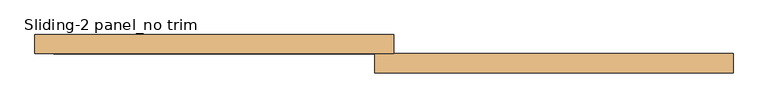
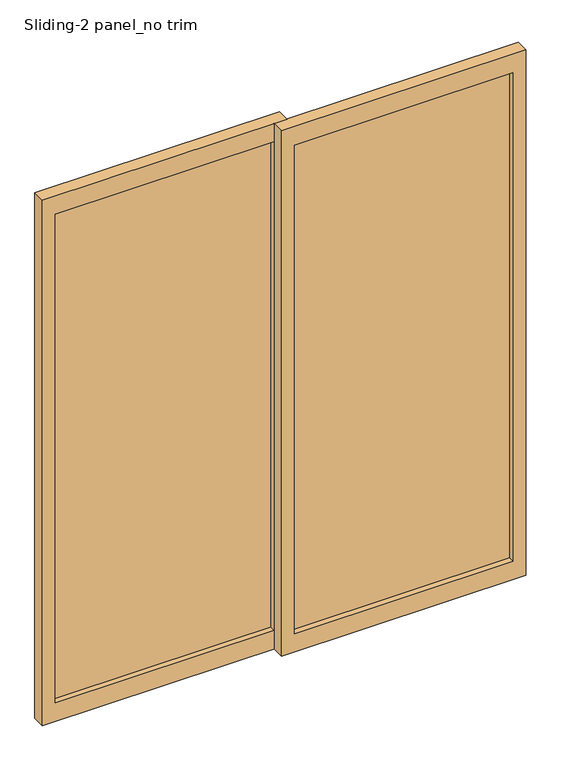
"""IFC4 building model written with IfcOpenShell, lengths in millimetres: door geometry, Sliding-2 panel_no trim."""

from ifc_helpers import new_model, si_unit, frame, origin, place, context, project, spatial, polyline, outline, extrude, source, transform, mapped, element, save


def sliding_2_panel_no_trim_2490c277(model_context):
    return source(origin(), model_context, "Body", "SweptSolid", [
        extrude(outline(polyline([(2133.996875, 25.4), (2133.996875, -914.9953125), (0.0, -914.9953125), (0.0, 25.4), (2133.996875, 25.4)]), holes=[polyline([(2058.9875, -24.60625), (75.009375, -24.60625), (75.009375, -864.9890625), (2058.9875, -864.9890625), (2058.9875, -24.60625)])]), frame((0.0, 191.99375, 0.0), z_axis=(0.0, 1.0, 0.0), x_axis=(0.0, 0.0, 1.0)), (0.0, 0.0, 1.0), 50.00625),
        extrude(outline(polyline([(2133.996875, 914.9953125), (2133.996875, -24.60625), (0.0, -24.60625), (0.0, 914.9953125), (2133.996875, 914.9953125)]), holes=[polyline([(2058.9875, 864.9890625), (75.009375, 864.9890625), (75.009375, 25.4), (2058.9875, 25.4), (2058.9875, 864.9890625)])]), frame((0.0, 141.9875, 0.0), z_axis=(0.0, 1.0, 0.0), x_axis=(0.0, 0.0, 1.0)), (0.0, 0.0, 1.0), 50.00625),
        extrude(outline(polyline([(-24.60625, 220.171875), (-24.60625, 213.821875), (-864.9890625, 213.821875), (-864.9890625, 220.171875), (-24.60625, 220.171875)])), frame((0.0, 0.0, 75.009375), z_axis=(0.0, 0.0, 1.0), x_axis=(1.0, 0.0, 0.0)), (0.0, 0.0, 1.0), 1983.978125),
        extrude(outline(polyline([(864.1953125, 170.165625), (864.1953125, 163.815625), (25.4, 163.815625), (25.4, 170.165625), (864.1953125, 170.165625)])), frame((0.0, 0.0, 75.009375), z_axis=(0.0, 0.0, 1.0), x_axis=(1.0, 0.0, 0.0)), (0.0, 0.0, 1.0), 1983.978125),
    ])


if __name__ == "__main__":
    model = new_model("IFC4")
    model_context = context("Model", 3, world=origin())
    ifc_project = project(units=[si_unit("LENGTHUNIT", "METRE", prefix="MILLI")], contexts=[model_context])
    site = spatial("IfcSite", under=ifc_project)
    building = spatial("IfcBuilding", under=site)
    placement = place(None, origin())
    sliding_2_panel_no_trim_shape = sliding_2_panel_no_trim_2490c277(model_context)
    element("IfcDoor", 1, ObjectType="Sliding-2 panel_no trim", at=placement, inside=building, context=model_context, shape_type="MappedRepresentation", body=[
        mapped(sliding_2_panel_no_trim_shape, transform((0.0, 0.0, 0.0), x_axis=(1.0, 0.0, 0.0), y_axis=(0.0, 1.0, 0.0), z_axis=(0.0, 0.0, 1.0))),
    ])
    save(model, "model.ifc")

# Revit data of these elements
# Type "Sliding-2 panel_no trim"
#   Type Mark = "45"
#   Thickness = 50.006 mm
#   Height = 2133.997 mm
#   Rail Width = 75.009 mm
#   Stile Width = 50.006 mm
#   Width = 1829.991 mm
#   Door Material = Door - Panel
#   Frame Material = Door - Frame
#   Function = (empty or 0)
#   Assembly Code = ""
#   Wall Closure = (empty or 0)
# Element 1 (IfcDoor, "Sliding-2 panel_no trim")
#   Materials on its faces: "Door - Panel", "Glass"
# Materials
#   "Door - Panel": class "Wood", colour RGB 114 82 51, transparency 0
#   "Door - Frame": colour RGB 153 76 43, transparency 0
#   "Glass": class "Glass", colour RGB 218 227 224, transparency 0.85, Description = "Soda Lime Glass", Cost = 0
